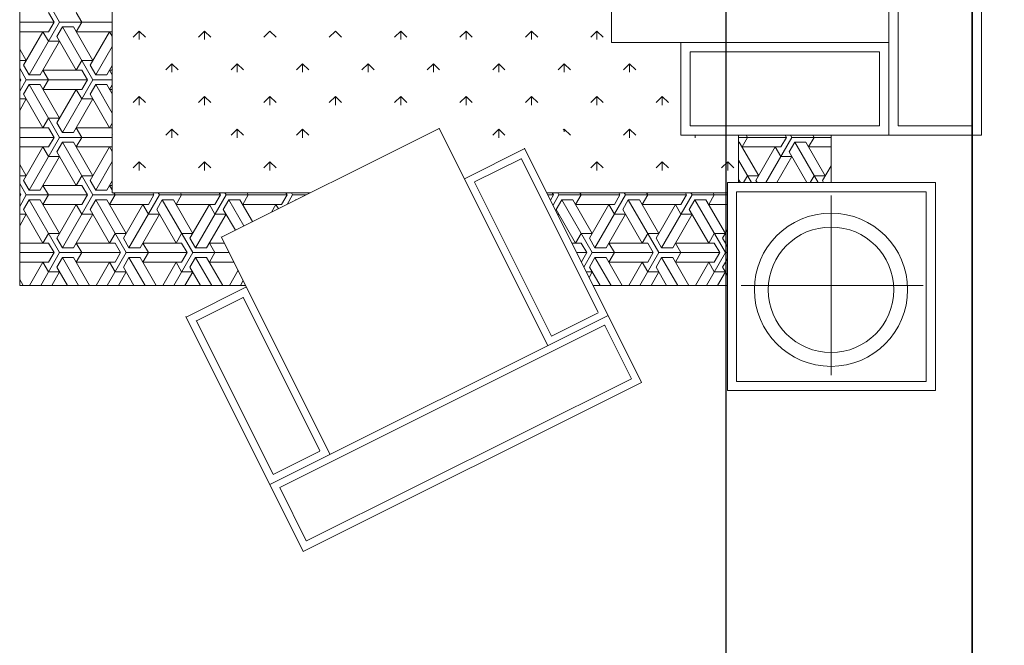
# Model space of a CAD drawing. Units: inches. Extents: x -1198 to -69, y -512 to 437.
# Tile 20 of 50: x -750 to -696, y 5 to 39. Entities that reach past the tile are written whole.
import ezdxf

# ---------------------------------------------------------------- set-up
doc = ezdxf.new("R2010")
doc.units = ezdxf.units.IN
doc.header["$MEASUREMENT"] = 0
for name, color, linetype, lineweight in [('A-ANNO-DIMS', 2, 'Continuous', 18), ('A-FURN', 60, 'Continuous', 18), ('A-WALL', 7, 'Continuous', 35)]:
    doc.layers.add(name, color=color, linetype=linetype, lineweight=lineweight)
doc.styles.get("Standard").update_dxf_attribs({"font": 'arial.ttf'})
doc.dimstyles.get("Standard").update_dxf_attribs({"dimtxt": 6, "dimasz": 6, "dimexe": 0.18, "dimexo": 0.0625, "dimgap": 0.09, "dimtad": 0, "dimtih": 1, "dimtoh": 1, "dimdec": 0, "dimzin": 0, "dimdsep": 46, "dimlunit": 4, "dimtxsty": 'Standard', "dimblk": 'OBLIQUE', "dimcen": 0.09, "dimadec": 0, "dimazin": 0, "dimtfac": 1, "dimtdec": 0, "dimtofl": 0, "dimtmove": 0, "dimatfit": 3, "dimfxl": 1, "dimtolj": 1, "dimtzin": 0, "dimarcsym": 0})

# ---------------------------------------------------------------- blocks, each defined once
blk = doc.blocks.new('A$C3B9F700E')
for p, q in [((736.9, 2080, -685.7), (2936.9, 2080, -685.7)), ((2936.9, 2080, -685.7), (2936.9, 1430, -685.7)), ((2936.9, 2080, -685.7), (2936.9, 1880, -685.7)), ((756.9, 2060, -685.7), (2916.9, 2060, -685.7)), ((2916.9, 2060, -685.7), (2916.9, 1900, -685.7)), ((3489.8, 1980.6, -685.7), (3039.8, 1980.6, -685.7)), ((3039.8, 1980.6, -685.7), (3039.8, 1530.6, -685.7)), ((3489.8, 1530.6, -685.7), (3489.8, 1980.6, -685.7)), ((3469.8, 1960.6, -685.7), (3059.8, 1960.6, -685.7)), ((3059.8, 1960.6, -685.7), (3059.8, 1550.6, -685.7)), ((3469.8, 1550.6, -685.7), (3469.8, 1960.6, -685.7)), ((3262.1, 1953.9, -685.7), (3262.1, 1560.5, -685.7)), ((2916.9, 1900, -685.7), (756.9, 1900, -685.7)), ((2936.9, 1880, -685.7), (736.9, 1880, -685.7)), ((2936.9, 1880, -685.7), (736.9, 1880, -685.7)), ((2736.9, 1880, -685.7), (2736.9, 1280, -685.7)), ((2736.9, 1430, -685.7), (2736.9, 1880, -685.7)), ((2736.9, 1880, -685.7), (2936.9, 1880, -685.7)), ((2936.9, 1880, -685.7), (2936.9, 1430, -685.7)), ((2756.9, 1450, -685.7), (2756.9, 1860, -685.7)), ((2756.9, 1860, -685.7), (2916.9, 1860, -685.7)), ((2916.9, 1860, -685.7), (2916.9, 1450, -685.7)), ((2936.9, 1754.8, -685.7), (3039.8, 1754.8, -685.7)), ((2936.9, 1554.8, -685.7), (2936.9, 1754.8, -685.7)), ((2936.9, 1754.8, -685.7), (3039.8, 1754.8, -685.7)), ((2941.9, 1670.3, -685.7), (2941.9, 1754.8, -685.7)), ((2962.7, 1754.8, -685.7), (2962.7, 1706.3, -685.7)), ((3035.5, 1736.3, -685.7), (3003.4, 1754.8, -685.7)), ((3039.8, 1754.8, -685.7), (3039.8, 1554.8, -685.7)), ((3456.2, 1754.8, -685.7), (3068, 1754.8, -685.7)), ((2952.3, 1700.3, -685.7), (3025.1, 1742.3, -685.7)), ((3039.8, 1726.8, -685.7), (2952.3, 1676.3, -685.7)), ((3025.1, 1718.3, -685.7), (3025.1, 1742.3, -685.7)), ((3039.8, 1738.8, -685.7), (3035.5, 1736.3, -685.7)), ((2941.9, 1718.3, -685.7), (2936.9, 1715.4, -685.7)), ((2941.9, 1718.3, -685.7), (2962.7, 1706.3, -685.7)), ((3025.1, 1718.3, -685.7), (3039.8, 1709.8, -685.7)), ((2952.3, 1676.3, -685.7), (2952.3, 1700.3, -685.7)), ((2973.1, 1664.3, -685.7), (3039.8, 1702.8, -685.7)), ((2941.9, 1670.3, -685.7), (2936.9, 1667.4, -685.7)), ((2941.9, 1670.3, -685.7), (3039.8, 1613.8, -685.7)), ((2952.3, 1676.3, -685.7), (2973.1, 1664.3, -685.7)), ((3039.8, 1637.8, -685.7), (2983.5, 1670.3, -685.7)), ((2983.5, 1646.3, -685.7), (2983.5, 1670.3, -685.7)), ((2941.9, 1658.3, -685.7), (2936.9, 1655.4, -685.7)), ((2941.9, 1658.3, -685.7), (2962.7, 1646.3, -685.7)), ((2941.9, 1554.8, -685.7), (2941.9, 1658.3, -685.7)), ((2962.7, 1646.3, -685.7), (2962.7, 1562.3, -685.7)), ((2983.5, 1646.3, -685.7), (2962.7, 1634.3, -685.7)), ((3035.5, 1592.3, -685.7), (2962.7, 1634.3, -685.7)), ((2952.3, 1556.3, -685.7), (3025.1, 1598.3, -685.7)), ((3025.1, 1574.3, -685.7), (3025.1, 1598.3, -685.7)), ((3039.8, 1582.8, -685.7), (2991.3, 1554.8, -685.7)), ((3039.8, 1594.8, -685.7), (3035.5, 1592.3, -685.7)), ((2941.9, 1574.3, -685.7), (2936.9, 1571.4, -685.7)), ((3039.8, 1554.8, -685.7), (2936.9, 1554.8, -685.7)), ((2936.9, 1554.8, -685.7), (3039.8, 1554.8, -685.7)), ((2941.9, 1574.3, -685.7), (2962.7, 1562.3, -685.7)), ((2952.3, 1554.8, -685.7), (2952.3, 1556.3, -685.7)), ((3025.1, 1574.3, -685.7), (3039.8, 1565.8, -685.7)), ((3032.8, 1554.8, -685.7), (3039.8, 1558.8, -685.7)), ((2994.6, 1531.3, -685.7), (3007.9, 1544.5, -685.7)), ((3059.8, 1550.6, -685.7), (3469.8, 1550.6, -685.7)), ((2994.6, 1531.3, -685.7), (3013.4, 1531.3, -685.7)), ((2994.6, 1531.3, -685.7), (3007.9, 1518, -685.7)), ((3039.8, 1530.6, -685.7), (3489.8, 1530.6, -685.7)), ((3062.1, 1140.2, -685.7), (3062.1, 1530.6, -685.7)), ((3062.1, 1530.6, -685.7), (3062.1, 1140.2, -685.7)), ((3062.1, 1530.6, -685.7), (3262.1, 1530.6, -685.7)), ((3066.6, 1454.3, -685.7), (3066.6, 1530.6, -685.7)), ((3077, 1484.3, -685.7), (3149.8, 1526.3, -685.7)), ((3191.3, 1526.3, -685.7), (3077, 1460.3, -685.7)), ((3087.4, 1530.6, -685.7), (3087.4, 1490.3, -685.7)), ((3160.2, 1520.3, -685.7), (3142.3, 1530.6, -685.7)), ((3149.8, 1502.3, -685.7), (3149.8, 1526.3, -685.7)), ((3178, 1530.6, -685.7), (3160.2, 1520.3, -685.7)), ((3191.3, 1514.3, -685.7), (3170.6, 1502.3, -685.7)), ((3191.3, 1526.3, -685.7), (3191.3, 1530.6, -685.7)), ((3191.3, 1526.3, -685.7), (3262.1, 1485.5, -685.7)), ((3191.3, 1382.3, -685.7), (3191.3, 1514.3, -685.7)), ((3191.3, 1514.3, -685.7), (3212.1, 1502.3, -685.7)), ((3204.7, 1530.6, -685.7), (3222.5, 1520.3, -685.7)), ((3222.5, 1520.3, -685.7), (3240.3, 1530.6, -685.7)), ((3262.1, 1509.5, -685.7), (3232.9, 1526.3, -685.7)), ((3232.9, 1502.3, -685.7), (3232.9, 1526.3, -685.7)), ((3262.1, 1530.6, -685.7), (3262.1, 1240.1, -685.7)), ((3262.1, 1530.6, -685.7), (3262.1, 1240.1, -685.7)), ((3066.6, 1502.3, -685.7), (3062.1, 1499.7, -685.7)), ((3066.6, 1502.3, -685.7), (3087.4, 1490.3, -685.7)), ((3149.8, 1502.3, -685.7), (3170.6, 1490.3, -685.7)), ((3170.6, 1502.3, -685.7), (3170.6, 1418.3, -685.7)), ((3212.1, 1502.3, -685.7), (3212.1, 1418.3, -685.7)), ((3232.9, 1502.3, -685.7), (3212.1, 1490.3, -685.7)), ((2936.9, 1473.6, -685.7), (2937.2, 1473.8, -685.7)), ((3077, 1460.3, -685.7), (3077, 1484.3, -685.7)), ((3097.8, 1448.3, -685.7), (3170.6, 1490.3, -685.7)), ((3262.1, 1461.5, -685.7), (3212.1, 1490.3, -685.7)), ((2916.9, 1450, -685.7), (2756.9, 1450, -685.7)), ((2936.9, 1460.6, -685.7), (2942.6, 1460.6, -685.7)), ((3066.6, 1454.3, -685.7), (3062.1, 1451.7, -685.7)), ((3066.6, 1454.3, -685.7), (3181, 1388.3, -685.7)), ((3077, 1460.3, -685.7), (3097.8, 1448.3, -685.7)), ((3181, 1412.3, -685.7), (3108.2, 1454.3, -685.7)), ((3108.2, 1430.3, -685.7), (3108.2, 1454.3, -685.7)), ((2936.9, 1430, -685.7), (2736.9, 1430, -685.7)), ((2936.9, 1430, -685.7), (2736.9, 1430, -685.7)), ((2936.9, 1447.6, -685.7), (2937.2, 1447.3, -685.7)), ((3066.6, 1442.3, -685.7), (3062.1, 1439.7, -685.7)), ((3066.6, 1310.3, -685.7), (3066.6, 1442.3, -685.7)), ((3066.6, 1442.3, -685.7), (3087.4, 1430.3, -685.7)), ((3087.4, 1430.3, -685.7), (3087.4, 1346.3, -685.7)), ((3108.2, 1430.3, -685.7), (3087.4, 1418.3, -685.7)), ((3191.3, 1430.3, -685.7), (3170.6, 1418.3, -685.7)), ((3191.3, 1430.3, -685.7), (3212.1, 1418.3, -685.7)), ((3201.7, 1412.3, -685.7), (3262.1, 1447.2, -685.7)), ((3160.2, 1376.3, -685.7), (3087.4, 1418.3, -685.7)), ((3181, 1388.3, -685.7), (3181, 1412.3, -685.7)), ((3262.1, 1423.2, -685.7), (3201.7, 1388.3, -685.7)), ((3201.7, 1388.3, -685.7), (3201.7, 1412.3, -685.7)), ((2853.2, 1389.9, -685.7), (2866.4, 1403.1, -685.7)), ((2853.2, 1389.9, -685.7), (2871.9, 1389.9, -685.7)), ((2853.2, 1389.9, -685.7), (2866.4, 1376.6, -685.7)), ((2994.6, 1389.9, -685.7), (3007.9, 1403.1, -685.7)), ((2994.6, 1389.9, -685.7), (3013.4, 1389.9, -685.7)), ((2994.6, 1389.9, -685.7), (3007.9, 1376.6, -685.7)), ((3181, 1388.3, -685.7), (3160.2, 1376.3, -685.7)), ((3201.7, 1388.3, -685.7), (3222.5, 1376.3, -685.7)), ((3222.5, 1376.3, -685.7), (3262.1, 1399.2, -685.7)), ((3077, 1340.3, -685.7), (3149.8, 1382.3, -685.7)), ((3191.3, 1382.3, -685.7), (3077, 1316.3, -685.7)), ((3149.8, 1358.3, -685.7), (3149.8, 1382.3, -685.7)), ((3191.3, 1370.3, -685.7), (3170.6, 1358.3, -685.7)), ((3191.3, 1382.3, -685.7), (3262.1, 1341.5, -685.7)), ((3191.3, 1370.3, -685.7), (3212.1, 1358.3, -685.7)), ((3191.3, 1238.3, -685.7), (3191.3, 1370.3, -685.7)), ((3262.1, 1365.5, -685.7), (3232.9, 1382.3, -685.7)), ((3232.9, 1358.3, -685.7), (3232.9, 1382.3, -685.7)), ((2965.3, 1091.9, -685.7), (3472.5, 1345.2, -685.7)), ((3066.6, 1358.3, -685.7), (3062.1, 1355.7, -685.7)), ((3066.6, 1358.3, -685.7), (3087.4, 1346.3, -685.7)), ((3097.8, 1304.3, -685.7), (3170.6, 1346.3, -685.7)), ((3149.8, 1358.3, -685.7), (3170.6, 1346.3, -685.7)), ((3170.6, 1358.3, -685.7), (3170.6, 1274.3, -685.7)), ((3212.1, 1358.3, -685.7), (3212.1, 1274.3, -685.7)), ((3232.9, 1358.3, -685.7), (3212.1, 1346.3, -685.7)), ((3262.1, 1317.5, -685.7), (3212.1, 1346.3, -685.7)), ((3472.5, 1345.2, -685.7), (3838, 613.2, -685.7)), ((2782.5, 1319.2, -685.7), (2795.7, 1332.4, -685.7)), ((2923.9, 1319.2, -685.7), (2937.2, 1332.4, -685.7)), ((3077, 1316.3, -685.7), (3077, 1340.3, -685.7)), ((3348.8, 1265.3, -685.7), (3464.4, 1323, -685.7)), ((3464.4, 1323, -685.7), (3815.2, 620.4, -685.7)), ((2782.5, 1319.2, -685.7), (2801.2, 1319.2, -685.7)), ((2782.5, 1319.2, -685.7), (2795.7, 1305.9, -685.7)), ((2923.9, 1319.2, -685.7), (2937.2, 1305.9, -685.7)), ((2923.9, 1319.2, -685.7), (2942.6, 1319.2, -685.7)), ((3066.6, 1310.3, -685.7), (3062.1, 1307.7, -685.7)), ((3066.6, 1310.3, -685.7), (3181, 1244.3, -685.7)), ((3077, 1316.3, -685.7), (3097.8, 1304.3, -685.7)), ((3181, 1268.3, -685.7), (3108.2, 1310.3, -685.7)), ((3108.2, 1286.3, -685.7), (3108.2, 1310.3, -685.7)), ((3201.7, 1268.3, -685.7), (3262.1, 1303.2, -685.7)), ((2736.9, 1280, -685.7), (936.9, 1280, -685.7)), ((3066.6, 1298.3, -685.7), (3062.1, 1295.7, -685.7)), ((3066.6, 1298.3, -685.7), (3087.4, 1286.3, -685.7)), ((3066.6, 1166.3, -685.7), (3066.6, 1298.3, -685.7)), ((3087.4, 1286.3, -685.7), (3087.4, 1202.3, -685.7)), ((3108.2, 1286.3, -685.7), (3087.4, 1274.3, -685.7)), ((3191.3, 1286.3, -685.7), (3170.6, 1274.3, -685.7)), ((3191.3, 1286.3, -685.7), (3212.1, 1274.3, -685.7)), ((3262.1, 1279.2, -685.7), (3201.7, 1244.3, -685.7)), ((2711.8, 1248.4, -685.7), (2725, 1261.7, -685.7)), ((2853.2, 1248.4, -685.7), (2866.4, 1261.7, -685.7)), ((2994.6, 1248.4, -685.7), (3007.9, 1261.7, -685.7)), ((3160.2, 1232.3, -685.7), (3087.4, 1274.3, -685.7)), ((3181, 1244.3, -685.7), (3181, 1268.3, -685.7)), ((3201.7, 1244.3, -685.7), (3201.7, 1268.3, -685.7)), ((3327.6, 1272.8, -685.7), (3693.1, 540.9, -685.7)), ((3348.6, 1264.7, -685.7), (3348.8, 1265.3, -685.7)), ((3699.2, 562.5, -685.7), (3348.6, 1264.7, -685.7)), ((2711.8, 1248.4, -685.7), (2725, 1235.2, -685.7)), ((2711.8, 1248.4, -685.7), (2730.5, 1248.4, -685.7)), ((2853.2, 1248.4, -685.7), (2866.4, 1235.2, -685.7)), ((2853.2, 1248.4, -685.7), (2871.9, 1248.4, -685.7)), ((2987.4, 1084.8, -685.7), (3320, 1250.9, -685.7)), ((2994.6, 1248.4, -685.7), (3007.9, 1235.2, -685.7)), ((2994.6, 1248.4, -685.7), (3013.4, 1248.4, -685.7)), ((3262.1, 1240.1, -685.7), (3062.1, 1140.2, -685.7)), ((3077, 1196.3, -685.7), (3149.8, 1238.3, -685.7)), ((3191.3, 1238.3, -685.7), (3077, 1172.3, -685.7)), ((3149.8, 1214.3, -685.7), (3149.8, 1238.3, -685.7)), ((3181, 1244.3, -685.7), (3160.2, 1232.3, -685.7)), ((3191.3, 1238.3, -685.7), (3222.5, 1220.3, -685.7)), ((3201.7, 1244.3, -685.7), (3222.5, 1232.3, -685.7)), ((3222.5, 1232.3, -685.7), (3262.1, 1255.2, -685.7)), ((3244.8, 1231.5, -685.7), (3232.9, 1238.3, -685.7)), ((3232.9, 1225.5, -685.7), (3232.9, 1238.3, -685.7)), ((3321.4, 1251.2, -685.7), (3371.9, 1150.1, -685.7)), ((3066.6, 1214.3, -685.7), (3062.1, 1211.7, -685.7)), ((3066.6, 1214.3, -685.7), (3087.4, 1202.3, -685.7)), ((3149.8, 1214.3, -685.7), (3170.6, 1202.3, -685.7)), ((3191.3, 1226.3, -685.7), (3170.6, 1214.3, -685.7)), ((3170.6, 1214.3, -685.7), (3170.6, 1194.4, -685.7)), ((3191.3, 1226.3, -685.7), (3211.4, 1214.8, -685.7)), ((3191.3, 1204.8, -685.7), (3191.3, 1226.3, -685.7)), ((3077, 1172.3, -685.7), (3077, 1196.3, -685.7)), ((3097.8, 1160.3, -685.7), (3170.6, 1202.3, -685.7)), ((2782.5, 1177.7, -685.7), (2795.7, 1191, -685.7)), ((2782.5, 1177.7, -685.7), (2801.2, 1177.7, -685.7)), ((2782.5, 1177.7, -685.7), (2795.7, 1164.5, -685.7)), ((2923.9, 1177.7, -685.7), (2937.2, 1191, -685.7)), ((2923.9, 1177.7, -685.7), (2925.9, 1175.7, -685.7)), ((2923.9, 1177.7, -685.7), (2930, 1177.7, -685.7)), ((3077, 1172.3, -685.7), (3097.8, 1160.3, -685.7)), ((3038.9, 983.8, -685.7), (3371.9, 1150.1, -685.7)), ((3066.6, 1166.3, -685.7), (3062.1, 1163.7, -685.7)), ((3066.6, 1154.3, -685.7), (3062.1, 1151.7, -685.7)), ((3066.6, 1166.3, -685.7), (3088.8, 1153.5, -685.7)), ((3066.6, 1154.3, -685.7), (3077.6, 1148, -685.7)), ((3066.6, 1142.5, -685.7), (3066.6, 1154.3, -685.7)), ((3111.1, 1164.7, -685.7), (3108.2, 1166.3, -685.7)), ((3108.2, 1163.2, -685.7), (3108.2, 1166.3, -685.7)), ((2921.7, 907.1, -685.7), (3392.7, 1142.3, -685.7)), ((2711.8, 1107, -685.7), (2725, 1120.3, -685.7)), ((2853.2, 1107, -685.7), (2866.4, 1120.3, -685.7)), ((2711.8, 1107, -685.7), (2725, 1093.8, -685.7)), ((2711.8, 1107, -685.7), (2730.5, 1107, -685.7)), ((2853.2, 1107, -685.7), (2866.4, 1093.8, -685.7)), ((2853.2, 1107, -685.7), (2871.9, 1107, -685.7)), ((2966.2, 1092.3, -685.7), (3031.3, 961.9, -685.7)), ((2988.1, 1084.7, -685.7), (3038.4, 984, -685.7)), ((2782.5, 1036.3, -685.7), (2795.7, 1049.6, -685.7)), ((2923.9, 1036.3, -685.7), (2937.2, 1049.6, -685.7)), ((2782.5, 1036.3, -685.7), (2801.2, 1036.3, -685.7)), ((2782.5, 1036.3, -685.7), (2795.7, 1023.1, -685.7)), ((2923.9, 1036.3, -685.7), (2937.2, 1023.1, -685.7)), ((2923.9, 1036.3, -685.7), (2942.6, 1036.3, -685.7)), ((2711.8, 965.6, -685.7), (2725, 978.9, -685.7)), ((2711.8, 965.6, -685.7), (2725, 952.3, -685.7)), ((2711.8, 965.6, -685.7), (2730.5, 965.6, -685.7)), ((2853.2, 965.6, -685.7), (2866.4, 978.9, -685.7)), ((2853.2, 965.6, -685.7), (2866.4, 952.3, -685.7)), ((2853.2, 965.6, -685.7), (2871.9, 965.6, -685.7)), ((2782.5, 894.9, -685.7), (2795.7, 908.1, -685.7)), ((2782.5, 894.9, -685.7), (2801.2, 894.9, -685.7)), ((2782.5, 894.9, -685.7), (2795.7, 881.6, -685.7)), ((2922.6, 907.6, -685.7), (3157.8, 436.6, -685.7)), ((2711.8, 824.2, -685.7), (2725, 837.4, -685.7)), ((2853.2, 824.2, -685.7), (2866.4, 837.4, -685.7)), ((2711.8, 824.2, -685.7), (2725, 810.9, -685.7)), ((2711.8, 824.2, -685.7), (2730.5, 824.2, -685.7)), ((2853.2, 824.2, -685.7), (2866.4, 810.9, -685.7)), ((2853.2, 824.2, -685.7), (2871.9, 824.2, -685.7)), ((2782.5, 753.5, -685.7), (2795.7, 766.7, -685.7)), ((2782.5, 753.5, -685.7), (2801.2, 753.5, -685.7)), ((2782.5, 753.5, -685.7), (2795.7, 740.2, -685.7)), ((2711.8, 682.8, -685.7), (2725, 696, -685.7)), ((2711.8, 682.8, -685.7), (2725, 669.5, -685.7)), ((2853.2, 682.8, -685.7), (2866.4, 696, -685.7)), ((2853.2, 682.8, -685.7), (2866.4, 669.5, -685.7)), ((2853.2, 682.8, -685.7), (2871.9, 682.8, -685.7)), ((3156.9, 436.1, -685.7), (3627.9, 671.3, -685.7)), ((3287.7, 483.3, -685.7), (3620.3, 649.4, -685.7)), ((3620.9, 649.2, -685.7), (3671.2, 548.5, -685.7)), ((2782.5, 612, -685.7), (2795.7, 625.3, -685.7)), ((2923.9, 612, -685.7), (2937.2, 625.3, -685.7)), ((3062.1, 628.3, -685.7), (3062.1, 200, -685.7)), ((3157.8, 436.6, -685.7), (3062.1, 628.3, -685.7)), ((3062.1, 628.3, -685.7), (3062.1, 200, -685.7)), ((3066.6, 590.3, -685.7), (3066.6, 619.2, -685.7)), ((3815, 619.9, -685.7), (3699.8, 562.3, -685.7)), ((3815.2, 620.4, -685.7), (3815, 619.9, -685.7)), ((2782.5, 612, -685.7), (2801.2, 612, -685.7)), ((2782.5, 612, -685.7), (2795.7, 598.8, -685.7)), ((2923.9, 612, -685.7), (2937.2, 598.8, -685.7)), ((2923.9, 612, -685.7), (2942.6, 612, -685.7)), ((3077, 596.3, -685.7), (3077, 598.3, -685.7)), ((3077.8, 596.8, -685.7), (3077, 596.3, -685.7)), ((3077, 596.3, -685.7), (3078.4, 595.5, -685.7)), ((3329.8, 359.5, -685.7), (3838, 613.2, -685.7)), ((3066.6, 590.3, -685.7), (3062.1, 587.7, -685.7)), ((3066.6, 578.3, -685.7), (3062.1, 575.7, -685.7)), ((3066.6, 590.3, -685.7), (3086.9, 578.6, -685.7)), ((3066.6, 578.3, -685.7), (3087.4, 566.3, -685.7)), ((3066.6, 446.3, -685.7), (3066.6, 578.3, -685.7)), ((2711.8, 541.3, -685.7), (2725, 554.6, -685.7)), ((2853.2, 541.3, -685.7), (2866.4, 554.6, -685.7)), ((2994.6, 541.3, -685.7), (3007.9, 554.6, -685.7)), ((3087.4, 566.3, -685.7), (3087.4, 482.3, -685.7)), ((3096.4, 559.5, -685.7), (3087.4, 554.3, -685.7)), ((3103.7, 544.9, -685.7), (3087.4, 554.3, -685.7)), ((3699.8, 562.3, -685.7), (3699.2, 562.5, -685.7)), ((2711.8, 541.3, -685.7), (2725, 528.1, -685.7)), ((2853.2, 541.3, -685.7), (2866.4, 528.1, -685.7)), ((2853.2, 541.3, -685.7), (2871.9, 541.3, -685.7)), ((2994.6, 541.3, -685.7), (3007.9, 528.1, -685.7)), ((2994.6, 541.3, -685.7), (3013.4, 541.3, -685.7)), ((3338.4, 381.8, -685.7), (3671, 547.9, -685.7)), ((3066.6, 494.3, -685.7), (3062.1, 491.7, -685.7)), ((3066.6, 494.3, -685.7), (3087.4, 482.3, -685.7)), ((3077, 476.3, -685.7), (3124.3, 503.6, -685.7)), ((3265.6, 490.4, -685.7), (3330.7, 359.9, -685.7)), ((2782.5, 470.6, -685.7), (2795.7, 483.9, -685.7)), ((2782.5, 470.6, -685.7), (2801.2, 470.6, -685.7)), ((2782.5, 470.6, -685.7), (2795.7, 457.4, -685.7)), ((2923.9, 470.6, -685.7), (2937.2, 483.9, -685.7)), ((2923.9, 470.6, -685.7), (2942.6, 470.6, -685.7)), ((2923.9, 470.6, -685.7), (2937.2, 457.4, -685.7)), ((3133.6, 485, -685.7), (3077, 452.3, -685.7)), ((3077, 452.3, -685.7), (3077, 476.3, -685.7)), ((3262.1, 488.6, -685.7), (3157.8, 436.6, -685.7)), ((3262.1, 453.5, -685.7), (3229.4, 472.3, -685.7)), ((3251.7, 483.5, -685.7), (3262.1, 477.5, -685.7)), ((3262.1, 0, -685.7), (3262.1, 488.6, -685.7)), ((3262.1, 488.6, -685.7), (3262.1, 0, -685.7)), ((3288.4, 483.2, -685.7), (3338.7, 382.5, -685.7)), ((3077, 452.3, -685.7), (3097.8, 440.3, -685.7)), ((3097.8, 440.3, -685.7), (3142.9, 466.4, -685.7)), ((3191.3, 374.3, -685.7), (3191.3, 453.3, -685.7)), ((3212.1, 463.7, -685.7), (3212.1, 410.3, -685.7)), ((3066.6, 446.3, -685.7), (3062.1, 443.7, -685.7)), ((3066.6, 434.3, -685.7), (3062.1, 431.7, -685.7)), ((3066.6, 446.3, -685.7), (3181, 380.3, -685.7)), ((3066.6, 434.3, -685.7), (3087.4, 422.3, -685.7)), ((3066.6, 302.3, -685.7), (3066.6, 434.3, -685.7)), ((3181, 404.3, -685.7), (3108.2, 446.3, -685.7)), ((3108.2, 422.3, -685.7), (3108.2, 446.3, -685.7)), ((3170.6, 442.9, -685.7), (3170.6, 410.3, -685.7)), ((3201.7, 404.3, -685.7), (3262.1, 439.2, -685.7)), ((2711.8, 399.9, -685.7), (2725, 413.2, -685.7)), ((2853.2, 399.9, -685.7), (2866.4, 413.2, -685.7)), ((2994.6, 399.9, -685.7), (3007.9, 413.2, -685.7)), ((3087.4, 422.3, -685.7), (3087.4, 338.3, -685.7)), ((3108.2, 422.3, -685.7), (3087.4, 410.3, -685.7)), ((3160.2, 368.3, -685.7), (3087.4, 410.3, -685.7)), ((3191.3, 422.3, -685.7), (3170.6, 410.3, -685.7)), ((3191.3, 422.3, -685.7), (3212.1, 410.3, -685.7)), ((3262.1, 415.2, -685.7), (3201.7, 380.3, -685.7)), ((2711.8, 399.9, -685.7), (2730.5, 399.9, -685.7)), ((2711.8, 399.9, -685.7), (2725, 386.7, -685.7)), ((2853.2, 399.9, -685.7), (2871.9, 399.9, -685.7)), ((2853.2, 399.9, -685.7), (2866.4, 386.7, -685.7)), ((2994.6, 399.9, -685.7), (3013.4, 399.9, -685.7)), ((2994.6, 399.9, -685.7), (3007.9, 386.7, -685.7)), ((3181, 380.3, -685.7), (3181, 404.3, -685.7)), ((3201.7, 380.3, -685.7), (3201.7, 404.3, -685.7)), ((3222.5, 368.3, -685.7), (3262.1, 391.2, -685.7)), ((3077, 332.3, -685.7), (3149.8, 374.3, -685.7)), ((3191.3, 374.3, -685.7), (3077, 308.3, -685.7)), ((3149.8, 350.3, -685.7), (3149.8, 374.3, -685.7)), ((3181, 380.3, -685.7), (3160.2, 368.3, -685.7)), ((3191.3, 362.3, -685.7), (3170.6, 350.3, -685.7)), ((3191.3, 374.3, -685.7), (3262.1, 333.5, -685.7)), ((3191.3, 362.3, -685.7), (3212.1, 350.3, -685.7)), ((3191.3, 230.3, -685.7), (3191.3, 362.3, -685.7)), ((3201.7, 380.3, -685.7), (3222.5, 368.3, -685.7)), ((3262.1, 357.5, -685.7), (3232.9, 374.3, -685.7)), ((3232.9, 350.3, -685.7), (3232.9, 374.3, -685.7)), ((2782.5, 329.2, -685.7), (2795.7, 342.5, -685.7)), ((2923.9, 329.2, -685.7), (2937.2, 342.5, -685.7)), ((3066.6, 350.3, -685.7), (3062.1, 347.7, -685.7)), ((3066.6, 350.3, -685.7), (3087.4, 338.3, -685.7)), ((3149.8, 350.3, -685.7), (3170.6, 338.3, -685.7)), ((3170.6, 350.3, -685.7), (3170.6, 266.3, -685.7)), ((3212.1, 350.3, -685.7), (3212.1, 266.3, -685.7)), ((3232.9, 350.3, -685.7), (3212.1, 338.3, -685.7)), ((2782.5, 329.2, -685.7), (2801.2, 329.2, -685.7)), ((2782.5, 329.2, -685.7), (2795.7, 315.9, -685.7)), ((2923.9, 329.2, -685.7), (2937.2, 315.9, -685.7)), ((2923.9, 329.2, -685.7), (2942.6, 329.2, -685.7)), ((3077, 308.3, -685.7), (3077, 332.3, -685.7)), ((3097.8, 296.3, -685.7), (3170.6, 338.3, -685.7)), ((3262.1, 309.5, -685.7), (3212.1, 338.3, -685.7)), ((3066.6, 302.3, -685.7), (3062.1, 299.7, -685.7)), ((3066.6, 302.3, -685.7), (3181, 236.3, -685.7)), ((3077, 308.3, -685.7), (3097.8, 296.3, -685.7)), ((3181, 260.3, -685.7), (3108.2, 302.3, -685.7)), ((3108.2, 278.3, -685.7), (3108.2, 302.3, -685.7)), ((3066.6, 290.3, -685.7), (3062.1, 287.7, -685.7)), ((3066.6, 290.3, -685.7), (3087.4, 278.3, -685.7)), ((3066.6, 158.3, -685.7), (3066.6, 290.3, -685.7)), ((3087.4, 278.3, -685.7), (3087.4, 194.3, -685.7)), ((3108.2, 278.3, -685.7), (3087.4, 266.3, -685.7)), ((3191.3, 278.3, -685.7), (3170.6, 266.3, -685.7)), ((3191.3, 278.3, -685.7), (3212.1, 266.3, -685.7)), ((3201.7, 260.3, -685.7), (3262.1, 295.2, -685.7)), ((2711.8, 258.5, -685.7), (2725, 271.8, -685.7)), ((2711.8, 258.5, -685.7), (2725, 245.2, -685.7)), ((2711.8, 258.5, -685.7), (2730.5, 258.5, -685.7)), ((2853.2, 258.5, -685.7), (2866.4, 271.8, -685.7)), ((2853.2, 258.5, -685.7), (2866.4, 245.2, -685.7)), ((2853.2, 258.5, -685.7), (2871.9, 258.5, -685.7)), ((2994.6, 258.5, -685.7), (3007.9, 271.8, -685.7)), ((2994.6, 258.5, -685.7), (3007.9, 245.2, -685.7)), ((2994.6, 258.5, -685.7), (3013.4, 258.5, -685.7)), ((3160.2, 224.3, -685.7), (3087.4, 266.3, -685.7)), ((3181, 236.3, -685.7), (3181, 260.3, -685.7)), ((3262.1, 271.2, -685.7), (3201.7, 236.3, -685.7)), ((3201.7, 236.3, -685.7), (3201.7, 260.3, -685.7)), ((3181, 236.3, -685.7), (3160.2, 224.3, -685.7)), ((3201.7, 236.3, -685.7), (3222.5, 224.3, -685.7)), ((3222.5, 224.3, -685.7), (3262.1, 247.2, -685.7)), ((3077, 188.3, -685.7), (3149.8, 230.3, -685.7)), ((3191.3, 230.3, -685.7), (3077, 164.3, -685.7)), ((3149.8, 206.3, -685.7), (3149.8, 230.3, -685.7)), ((3191.3, 218.3, -685.7), (3170.6, 206.3, -685.7)), ((3191.3, 230.3, -685.7), (3262.1, 189.5, -685.7)), ((3191.3, 218.3, -685.7), (3212.1, 206.3, -685.7)), ((3191.3, 86.3, -685.7), (3191.3, 218.3, -685.7)), ((3262.1, 213.5, -685.7), (3232.9, 230.3, -685.7)), ((3232.9, 206.3, -685.7), (3232.9, 230.3, -685.7)), ((3062.1, 200, -685.7), (601.4, 200, -685.7)), ((3062.1, 200, -685.7), (601.4, 200, -685.7)), ((2692.5, 86.3, -685.7), (2692.5, 200, -685.7)), ((2713.3, 200, -685.7), (2713.3, 122.3, -685.7)), ((2723.1, 200, -685.7), (2713.3, 194.3, -685.7)), ((2786, 152.3, -685.7), (2713.3, 194.3, -685.7)), ((2745, 200, -685.7), (2806.8, 164.3, -685.7)), ((2806.8, 188.3, -685.7), (2786.6, 200, -685.7)), ((2794.7, 200, -685.7), (2795.7, 201, -685.7)), ((2796.4, 200, -685.7), (2796.4, 194.3, -685.7)), ((2806.3, 200, -685.7), (2796.4, 194.3, -685.7)), ((2817.2, 158.3, -685.7), (2817.2, 200, -685.7)), ((2827.6, 188.3, -685.7), (2847.8, 200, -685.7)), ((2889.4, 200, -685.7), (2827.6, 164.3, -685.7)), ((2828.2, 200, -685.7), (2838, 194.3, -685.7)), ((2838, 200, -685.7), (2838, 194.3, -685.7)), ((2848.4, 152.3, -685.7), (2921.1, 194.3, -685.7)), ((2911.3, 200, -685.7), (2921.1, 194.3, -685.7)), ((2921.1, 200, -685.7), (2921.1, 122.3, -685.7)), ((2936.1, 200, -685.7), (2937.2, 201, -685.7)), ((2941.9, 86.3, -685.7), (2941.9, 200, -685.7)), ((2962.7, 200, -685.7), (2962.7, 122.3, -685.7)), ((2972.5, 200, -685.7), (2962.7, 194.3, -685.7)), ((3035.5, 152.3, -685.7), (2962.7, 194.3, -685.7)), ((2994.4, 200, -685.7), (3056.2, 164.3, -685.7)), ((3056.2, 188.3, -685.7), (3036, 200, -685.7)), ((3045.9, 200, -685.7), (3045.9, 194.3, -685.7)), ((3055.7, 200, -685.7), (3045.9, 194.3, -685.7)), ((3066.6, 206.3, -685.7), (3062.1, 203.7, -685.7)), ((3066.6, 206.3, -685.7), (3087.4, 194.3, -685.7)), ((3097.8, 152.3, -685.7), (3170.6, 194.3, -685.7)), ((3149.8, 206.3, -685.7), (3170.6, 194.3, -685.7)), ((3170.6, 206.3, -685.7), (3170.6, 122.3, -685.7)), ((3212.1, 206.3, -685.7), (3212.1, 122.3, -685.7)), ((3232.9, 206.3, -685.7), (3212.1, 194.3, -685.7)), ((3262.1, 165.5, -685.7), (3212.1, 194.3, -685.7)), ((2806.8, 164.3, -685.7), (2806.8, 188.3, -685.7)), ((2827.6, 164.3, -685.7), (2827.6, 188.3, -685.7)), ((3056.2, 164.3, -685.7), (3056.2, 188.3, -685.7)), ((3077, 164.3, -685.7), (3077, 188.3, -685.7)), ((2702.9, 116.3, -685.7), (2775.7, 158.3, -685.7)), ((2817.2, 158.3, -685.7), (2702.9, 92.3, -685.7)), ((2775.7, 134.3, -685.7), (2775.7, 158.3, -685.7)), ((2806.8, 164.3, -685.7), (2786, 152.3, -685.7)), ((2817.2, 158.3, -685.7), (2931.5, 92.3, -685.7)), ((2827.6, 164.3, -685.7), (2848.4, 152.3, -685.7)), ((2931.5, 116.3, -685.7), (2858.8, 158.3, -685.7)), ((2858.8, 134.3, -685.7), (2858.8, 158.3, -685.7)), ((2952.3, 116.3, -685.7), (3025.1, 158.3, -685.7)), ((3066.6, 158.3, -685.7), (2952.3, 92.3, -685.7)), ((3025.1, 134.3, -685.7), (3025.1, 158.3, -685.7)), ((3056.2, 164.3, -685.7), (3035.5, 152.3, -685.7)), ((3066.6, 158.3, -685.7), (3181, 92.3, -685.7)), ((3077, 164.3, -685.7), (3097.8, 152.3, -685.7)), ((3181, 116.3, -685.7), (3108.2, 158.3, -685.7)), ((3108.2, 134.3, -685.7), (3108.2, 158.3, -685.7)), ((3201.7, 116.3, -685.7), (3262.1, 151.2, -685.7)), ((2692.5, 134.3, -685.7), (2671.7, 122.3, -685.7)), ((2692.5, 134.3, -685.7), (2713.3, 122.3, -685.7)), ((2775.7, 134.3, -685.7), (2796.4, 122.3, -685.7)), ((2817.2, 146.3, -685.7), (2796.4, 134.3, -685.7)), ((2796.4, 134.3, -685.7), (2796.4, 50.3, -685.7)), ((2817.2, 146.3, -685.7), (2838, 134.3, -685.7)), ((2817.2, 14.3, -685.7), (2817.2, 146.3, -685.7)), ((2838, 134.3, -685.7), (2838, 50.3, -685.7)), ((2858.8, 134.3, -685.7), (2838, 122.3, -685.7)), ((2941.9, 134.3, -685.7), (2921.1, 122.3, -685.7)), ((2941.9, 134.3, -685.7), (2962.7, 122.3, -685.7)), ((3025.1, 134.3, -685.7), (3045.9, 122.3, -685.7)), ((3066.6, 146.3, -685.7), (3045.9, 134.3, -685.7)), ((3045.9, 134.3, -685.7), (3045.9, 50.3, -685.7)), ((3066.6, 146.3, -685.7), (3087.4, 134.3, -685.7)), ((3066.6, 14.3, -685.7), (3066.6, 146.3, -685.7)), ((3087.4, 134.3, -685.7), (3087.4, 50.3, -685.7)), ((3108.2, 134.3, -685.7), (3087.4, 122.3, -685.7)), ((3191.3, 134.3, -685.7), (3170.6, 122.3, -685.7)), ((3191.3, 134.3, -685.7), (3212.1, 122.3, -685.7)), ((2702.9, 92.3, -685.7), (2702.9, 116.3, -685.7)), ((2723.7, 80.3, -685.7), (2796.4, 122.3, -685.7)), ((2910.8, 80.3, -685.7), (2838, 122.3, -685.7)), ((2931.5, 92.3, -685.7), (2931.5, 116.3, -685.7)), ((2952.3, 92.3, -685.7), (2952.3, 116.3, -685.7)), ((2973.1, 80.3, -685.7), (3045.9, 122.3, -685.7)), ((3160.2, 80.3, -685.7), (3087.4, 122.3, -685.7)), ((3181, 92.3, -685.7), (3181, 116.3, -685.7)), ((3262.1, 127.2, -685.7), (3201.7, 92.3, -685.7)), ((3201.7, 92.3, -685.7), (3201.7, 116.3, -685.7)), ((2692.5, 86.3, -685.7), (2578.2, 20.3, -685.7)), ((2692.5, 86.3, -685.7), (2806.8, 20.3, -685.7)), ((2702.9, 92.3, -685.7), (2723.7, 80.3, -685.7)), ((2806.8, 44.3, -685.7), (2734.1, 86.3, -685.7)), ((2734.1, 62.3, -685.7), (2734.1, 86.3, -685.7)), ((2827.6, 44.3, -685.7), (2900.4, 86.3, -685.7)), ((2941.9, 86.3, -685.7), (2827.6, 20.3, -685.7)), ((2900.4, 62.3, -685.7), (2900.4, 86.3, -685.7)), ((2931.5, 92.3, -685.7), (2910.8, 80.3, -685.7)), ((2941.9, 86.3, -685.7), (3056.2, 20.3, -685.7)), ((2952.3, 92.3, -685.7), (2973.1, 80.3, -685.7)), ((2983.5, 62.3, -685.7), (2983.5, 86.3, -685.7)), ((3056.2, 44.3, -685.7), (2983.5, 86.3, -685.7)), ((3077, 44.3, -685.7), (3149.8, 86.3, -685.7)), ((3191.3, 86.3, -685.7), (3077, 20.3, -685.7)), ((3149.8, 62.3, -685.7), (3149.8, 86.3, -685.7)), ((3181, 92.3, -685.7), (3160.2, 80.3, -685.7)), ((3191.3, 86.3, -685.7), (3262.1, 45.5, -685.7)), ((3201.7, 92.3, -685.7), (3222.5, 80.3, -685.7)), ((3222.5, 80.3, -685.7), (3262.1, 103.2, -685.7)), ((3262.1, 69.5, -685.7), (3232.9, 86.3, -685.7)), ((3232.9, 62.3, -685.7), (3232.9, 86.3, -685.7)), ((2692.5, 74.3, -685.7), (2671.7, 62.3, -685.7)), ((2692.5, 74.3, -685.7), (2713.3, 62.3, -685.7)), ((2692.5, 0, -685.7), (2692.5, 74.3, -685.7)), ((2941.9, 74.3, -685.7), (2921.1, 62.3, -685.7)), ((2941.9, 74.3, -685.7), (2962.7, 62.3, -685.7)), ((2941.9, 0, -685.7), (2941.9, 74.3, -685.7)), ((3191.3, 74.3, -685.7), (3170.6, 62.3, -685.7)), ((3191.3, 74.3, -685.7), (3212.1, 62.3, -685.7)), ((3191.3, 0, -685.7), (3191.3, 74.3, -685.7)), ((2713.3, 62.3, -685.7), (2713.3, 0, -685.7)), ((2734.1, 62.3, -685.7), (2713.3, 50.3, -685.7)), ((2786, 8.3, -685.7), (2713.3, 50.3, -685.7)), ((2817.2, 62.3, -685.7), (2796.4, 50.3, -685.7)), ((2806.8, 20.3, -685.7), (2806.8, 44.3, -685.7)), ((2817.2, 62.3, -685.7), (2838, 50.3, -685.7)), ((2827.6, 20.3, -685.7), (2827.6, 44.3, -685.7)), ((2848.4, 8.3, -685.7), (2921.1, 50.3, -685.7)), ((2900.4, 62.3, -685.7), (2921.1, 50.3, -685.7)), ((2921.1, 62.3, -685.7), (2921.1, 0, -685.7)), ((2962.7, 62.3, -685.7), (2962.7, 0, -685.7)), ((2983.5, 62.3, -685.7), (2962.7, 50.3, -685.7)), ((3035.5, 8.3, -685.7), (2962.7, 50.3, -685.7)), ((3066.6, 62.3, -685.7), (3045.9, 50.3, -685.7)), ((3056.2, 20.3, -685.7), (3056.2, 44.3, -685.7)), ((3066.6, 62.3, -685.7), (3087.4, 50.3, -685.7)), ((3077, 20.3, -685.7), (3077, 44.3, -685.7)), ((3097.8, 8.3, -685.7), (3170.6, 50.3, -685.7)), ((3149.8, 62.3, -685.7), (3170.6, 50.3, -685.7)), ((3170.6, 62.3, -685.7), (3170.6, 0, -685.7)), ((3212.1, 62.3, -685.7), (3212.1, 0, -685.7)), ((3232.9, 62.3, -685.7), (3212.1, 50.3, -685.7)), ((3262.1, 21.5, -685.7), (3212.1, 50.3, -685.7)), ((401.4, 0, -685.7), (3262.1, 0, -685.7)), ((3262.1, 0, -685.7), (401.4, 0, -685.7)), ((2750.8, 0, -685.7), (2775.7, 14.3, -685.7)), ((2775.7, 0, -685.7), (2775.7, 14.3, -685.7)), ((2806.8, 20.3, -685.7), (2786, 8.3, -685.7)), ((2817.2, 14.3, -685.7), (2792.4, 0, -685.7)), ((2817.2, 2.3, -685.7), (2813.2, 0, -685.7)), ((2817.2, 14.3, -685.7), (2842, 0, -685.7)), ((2817.2, 2.3, -685.7), (2821.2, 0, -685.7)), ((2817.2, 0, -685.7), (2817.2, 2.3, -685.7)), ((2827.6, 20.3, -685.7), (2848.4, 8.3, -685.7)), ((2883.6, 0, -685.7), (2858.8, 14.3, -685.7)), ((2858.8, 0, -685.7), (2858.8, 14.3, -685.7)), ((3000.3, 0, -685.7), (3025.1, 14.3, -685.7)), ((3025.1, 0, -685.7), (3025.1, 14.3, -685.7)), ((3056.2, 20.3, -685.7), (3035.5, 8.3, -685.7)), ((3066.6, 14.3, -685.7), (3041.8, 0, -685.7)), ((3066.6, 2.3, -685.7), (3062.6, 0, -685.7)), ((3066.6, 14.3, -685.7), (3091.4, 0, -685.7)), ((3066.6, 2.3, -685.7), (3070.7, 0, -685.7)), ((3066.6, 0, -685.7), (3066.6, 2.3, -685.7)), ((3077, 20.3, -685.7), (3097.8, 8.3, -685.7)), ((3133, 0, -685.7), (3108.2, 14.3, -685.7)), ((3108.2, 0, -685.7), (3108.2, 14.3, -685.7)), ((3249.7, 0, -685.7), (3262.1, 7.2, -685.7))]:
    blk.add_line(p, q)
for radius in [165.7, 135.7]:
    blk.add_circle((3271.7, 1754.8, -685.7), radius)
blk = doc.blocks.new('1')
blk.add_blockref('A$C3B9F700E', (-1861.1, 172.7, 685.7))
blk = doc.blocks.new('_Oblique')
at = {"color": 0, "linetype": 'ByBlock', "lineweight": -2}
blk.add_line((-0.5, -0.5), (0.5, 0.5), dxfattribs=at)
blk = doc.blocks.new('*D76')
at = {"layer": 'A-ANNO-DIMS', "color": 0, "lineweight": -2, "ltscale": 10, "transparency": 16777216}
for p, q in [((-711.132, -38.21), (-711.132, 433.184)), ((-711.132, 433.004), (-697.751, 433.004)), ((-697.751, -38.21), (-697.751, 433.184)), ((-697.751, 433.004), (-691.751, 433.004))]:
    blk.add_line(p, q, dxfattribs=at)
at = {"layer": 'DEFPOINTS', "color": 0, "ltscale": 10, "transparency": 16777216}
for p in [(-697.751, 433.004), (-711.132, -38.272), (-697.751, -38.272)]:
    blk.add_point(p, dxfattribs=at)
at = {"layer": 'A-ANNO-DIMS', "color": 0, "lineweight": -2, "ltscale": 10, "transparency": 16777216, "xscale": 6, "yscale": 6, "zscale": 6, "rotation": 180}
blk.add_blockref('_Oblique', (-711.132, 433.004), dxfattribs=at)
at = {"layer": 'A-ANNO-DIMS', "color": 0, "lineweight": -2, "ltscale": 10, "transparency": 16777216, "xscale": 6, "yscale": 6, "zscale": 6}
blk.add_blockref('_Oblique', (-697.751, 433.004), dxfattribs=at)
at = {"layer": 'A-ANNO-DIMS', "color": 0, "ltscale": 10, "transparency": 16777216, "insert": (-681.814, 433.004), "char_height": 6, "attachment_point": 5}
blk.add_mtext('\\A1;13.38', dxfattribs=at)

msp = doc.modelspace()

# ---------------------------------------------------------------- linework, layer by layer
at = {"layer": 'A-WALL', "ltscale": 10}
for p, q in [((-697.7509, 158.2277), (-697.7509, 35.2277)), ((-697.7509, 35.2277), (-697.7509, -38.2723))]:
    msp.add_line(p, q, dxfattribs=at)

# ---------------------------------------------------------------- block references
at = {"layer": 'A-FURN', "ltscale": 10, "xscale": 0.0251614738227896, "yscale": 0.0251614738227896, "zscale": 0.0251614738227896, "rotation": 270.0000000000001}
msp.add_blockref('1', (-753.9284, 59.7223), dxfattribs=at)

# ---------------------------------------------------------------- dimensions: what is measured, and where the dimension line sits
at = {"layer": 'A-ANNO-DIMS', "ltscale": 10}
dim = msp.add_linear_dim(base=(-697.7509, 433.0036), p1=(-711.1319, -38.2723), p2=(-697.7509, -38.2723), dimstyle='Standard', override={"dimdec": 2, "dimlfac": 1, "dimrnd": 0, "dimzin": 0, "dimdsep": 46, "dimlunit": 2}, dxfattribs=at)
dim.commit()
dim.dimension.update_dxf_attribs({"geometry": '*D76', "text_midpoint": (-681.8137, 433.0036)})

doc.saveas('drawing.dxf')
